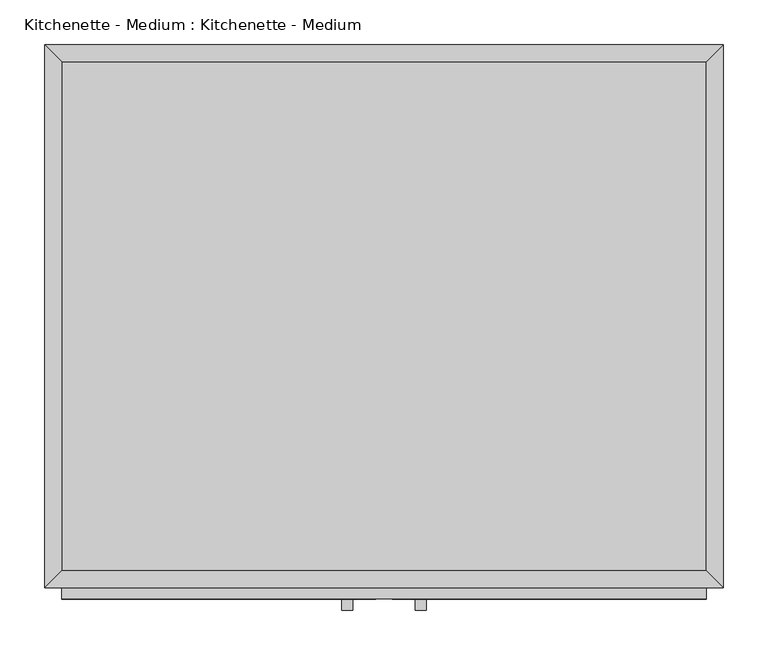
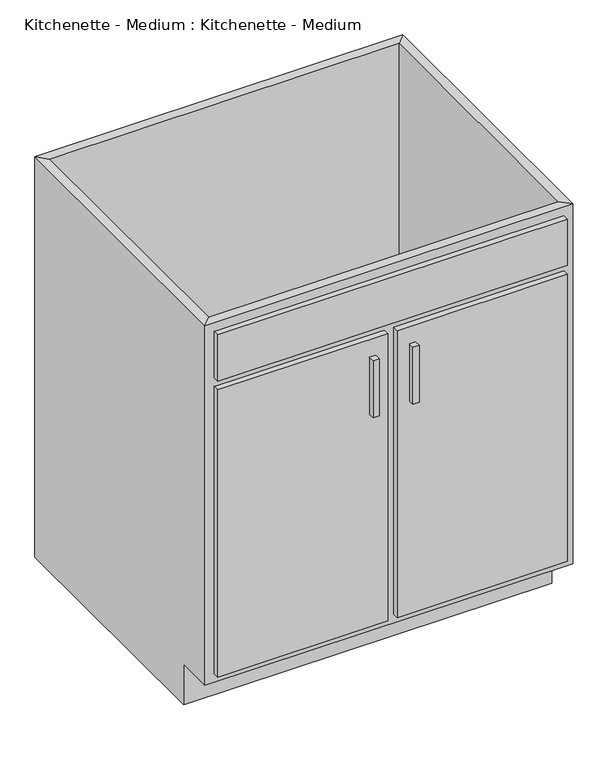
"""IFC4 building model written with IfcOpenShell, lengths in millimetres: proxy geometry, Kitchenette - Medium : Kitchenette - Medium."""

from ifc_helpers import new_model, si_unit, frame, origin, place, context, project, spatial, polyline, outline, extrude, faceted_brep, source, transform, mapped, element, save


def kitchenette_medium_kitchenette_medium_5bfe328f(model_context):
    return source(origin(), model_context, "Body", "SolidModel", [
        faceted_brep([(380.6877049, -590.55, 876.3), (380.6877049, -590.55, 88.9), (-343.2122951, -590.55, 88.9), (-343.2122951, -590.55, 876.3), (-362.2622951, -609.6, 876.3), (399.7377049, -609.6, 876.3), (-362.2622951, -609.6, 88.9), (399.7377049, -609.6, 88.9), (-343.2122951, -533.4, 88.9), (-343.2122951, -19.05, 88.9), (-343.2122951, -19.05, 876.3), (-362.2622951, 0.0, 876.3), (-362.2622951, 0.0, 0.0), (-362.2622951, -533.4, 0.0), (-362.2622951, -533.4, 88.9), (380.6877049, -19.05, 88.9), (380.6877049, -19.05, 876.3), (399.7377049, 0.0, 876.3), (399.7377049, 0.0, 0.0), (380.6877049, -533.4, 88.9), (399.7377049, -533.4, 88.9), (399.7377049, -533.4, 0.0)], [[[0, 1, 2, 3]], [[0, 3, 4, 5]], [[5, 4, 6, 7]], [[2, 1, 7, 6]], [[3, 2, 8, 9, 10]], [[4, 3, 10, 11]], [[6, 4, 11, 12, 13, 14]], [[2, 6, 14, 8]], [[10, 9, 15, 16]], [[11, 10, 16, 17]], [[12, 11, 17, 18]], [[1, 0, 16, 15, 19]], [[0, 5, 17, 16]], [[5, 7, 20, 21, 18, 17]], [[7, 1, 19, 20]], [[8, 19, 15, 9]], [[18, 21, 13, 12]], [[13, 21, 20, 19, 8, 14]]]),
        extrude(outline(polyline([(-16.1872951, -635.0), (-28.8872951, -635.0), (-28.8872951, -622.3), (-16.1872951, -622.3), (-16.1872951, -635.0)])), frame((0.0, 0.0, 573.769895), z_axis=(0.0, 0.0, 1.0), x_axis=(1.0, 0.0, 0.0)), (0.0, 0.0, 1.0), 124.730105),
        extrude(outline(polyline([(66.3627049, -635.0), (53.6627049, -635.0), (53.6627049, -622.3), (66.3627049, -622.3), (66.3627049, -635.0)])), frame((0.0, 0.0, 573.769895), z_axis=(0.0, 0.0, 1.0), x_axis=(1.0, 0.0, 0.0)), (0.0, 0.0, 1.0), 124.730105),
        extrude(outline(polyline([(380.6877049, -19.05), (380.6877049, -590.55), (-343.2122951, -590.55), (-343.2122951, -19.05), (380.6877049, -19.05)])), frame((0.0, 0.0, 88.9), z_axis=(0.0, 0.0, 1.0), x_axis=(1.0, 0.0, 0.0)), (0.0, 0.0, 1.0), 19.05),
        extrude(outline(polyline([(9.2127049, -622.3), (-343.2122951, -622.3), (-343.2122951, -609.6), (9.2127049, -609.6), (9.2127049, -622.3)])), frame((0.0, 0.0, 107.95), z_axis=(0.0, 0.0, 1.0), x_axis=(1.0, 0.0, 0.0)), (0.0, 0.0, 1.0), 628.65),
        extrude(outline(polyline([(380.6877049, -622.3), (28.2627049, -622.3), (28.2627049, -609.6), (380.6877049, -609.6), (380.6877049, -622.3)])), frame((0.0, 0.0, 107.95), z_axis=(0.0, 0.0, 1.0), x_axis=(1.0, 0.0, 0.0)), (0.0, 0.0, 1.0), 628.65),
        extrude(outline(polyline([(380.6877049, -622.3), (-343.2122951, -622.3), (-343.2122951, -609.6), (380.6877049, -609.6), (380.6877049, -622.3)])), frame((0.0, 0.0, 755.65), z_axis=(0.0, 0.0, 1.0), x_axis=(1.0, 0.0, 0.0)), (0.0, 0.0, 1.0), 101.6),
    ])


if __name__ == "__main__":
    model = new_model("IFC4")
    model_context = context("Model", 3, world=origin())
    ifc_project = project(units=[si_unit("LENGTHUNIT", "METRE", prefix="MILLI")], contexts=[model_context])
    site = spatial("IfcSite", under=ifc_project)
    building = spatial("IfcBuilding", under=site)
    placement = place(None, origin())
    kitchenette_medium_kitchenette_medium_shape = kitchenette_medium_kitchenette_medium_5bfe328f(model_context)
    element("IfcBuildingElementProxy", 1, Name="Kitchenette - Medium : Kitchenette - Medium", ObjectType="Kitchenette - Medium : Kitchenette - Medium", at=placement, inside=building, context=model_context, shape_type="MappedRepresentation", body=[
        mapped(kitchenette_medium_kitchenette_medium_shape, transform((0.0, 0.0, 0.0), x_axis=(1.0, 0.0, 0.0), y_axis=(0.0, 1.0, 0.0), z_axis=(0.0, 0.0, 1.0))),
    ])
    save(model, "model.ifc")

# Revit data of these elements
# Type "Kitchenette - Medium : Kitchenette - Medium"
#   Assembly Code = "E1090400"
#   Counter Length = 4' - 0"
#   Cabinet Width = 2' - 6"
#   Cabinet Height = 2' - 10 1/2"
#   Cabinet Depth = 2' - 0"
#   Toe Depth = 0' - 3"
#   Toe Height = 0' - 3 1/2"
#   Cabinet Material = Cabinets
#   Door/Drawer Material = Cabinets
#   Handle Material = Cabinets - Handles
#   Default Elevation = 0
# Element 1 (IfcBuildingElementProxy, "Kitchenette - Medium : Kitchenette - Medium")
#   Materials on its faces: "Cabinets", "Cabinets - Handles"
# Materials
#   "Cabinets": colour RGB 249 249 249, transparency 0
#   "Cabinets - Handles": class "Metal", colour RGB 57 57 57, transparency 0
